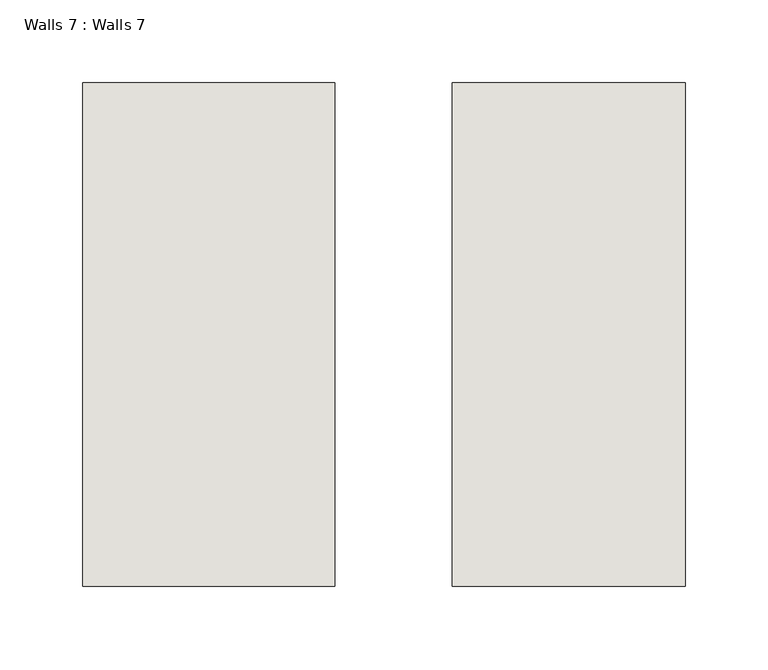
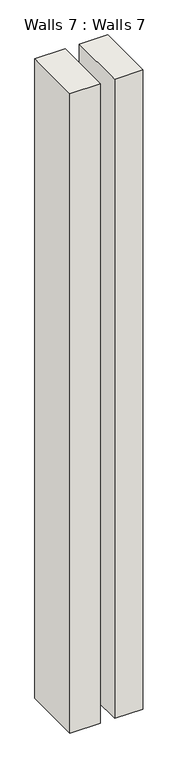
"""IFC4 building model written with IfcOpenShell, lengths in millimetres: wall geometry, Walls 7 : Walls 7."""

from ifc_helpers import new_model, si_unit, origin, origin_with_axes, place, context, project, spatial, polyline, outline, extrude, source, transform, mapped, element, save


def walls_7_walls_7_91501f10(model_context):
    return source(origin(), model_context, "Body", "SweptSolid", [
        extrude(outline(polyline([(-12329.6424966, 401.1257411), (-12329.6424966, 96.3257411), (-12482.0424966, 96.3257411), (-12482.0424966, 401.1257411), (-12329.6424966, 401.1257411)])), origin_with_axes(), (0.0, 0.0, 1.0), 3391.5795043),
        extrude(outline(polyline([(-12117.3437624, 401.1257411), (-12117.3437624, 96.3257411), (-12258.517466, 96.3257411), (-12258.517466, 401.1257411), (-12117.3437624, 401.1257411)])), origin_with_axes(), (0.0, 0.0, 1.0), 3391.5795043),
    ])


if __name__ == "__main__":
    model = new_model("IFC4")
    model_context = context("Model", 3, world=origin())
    ifc_project = project(units=[si_unit("LENGTHUNIT", "METRE", prefix="MILLI")], contexts=[model_context])
    site = spatial("IfcSite", under=ifc_project)
    building = spatial("IfcBuilding", under=site)
    placement = place(None, origin())
    walls_7_walls_7_shape = walls_7_walls_7_91501f10(model_context)
    element("IfcWall", 1, ObjectType="Walls 7 : Walls 7", at=placement, inside=building, context=model_context, shape_type="MappedRepresentation", body=[
        mapped(walls_7_walls_7_shape, transform((0.0, 0.0, 0.0), x_axis=(1.0, 0.0, 0.0), y_axis=(0.0, 1.0, 0.0), z_axis=(0.0, 0.0, 1.0))),
    ])
    save(model, "model.ifc")

# Revit data of these elements
# Element 1 (IfcWall, "Walls 7 : Walls 7")
#   Materials on its faces: "Default Wall"
# Materials
#   "Default Wall": colour RGB 128 128 128, transparency 0
